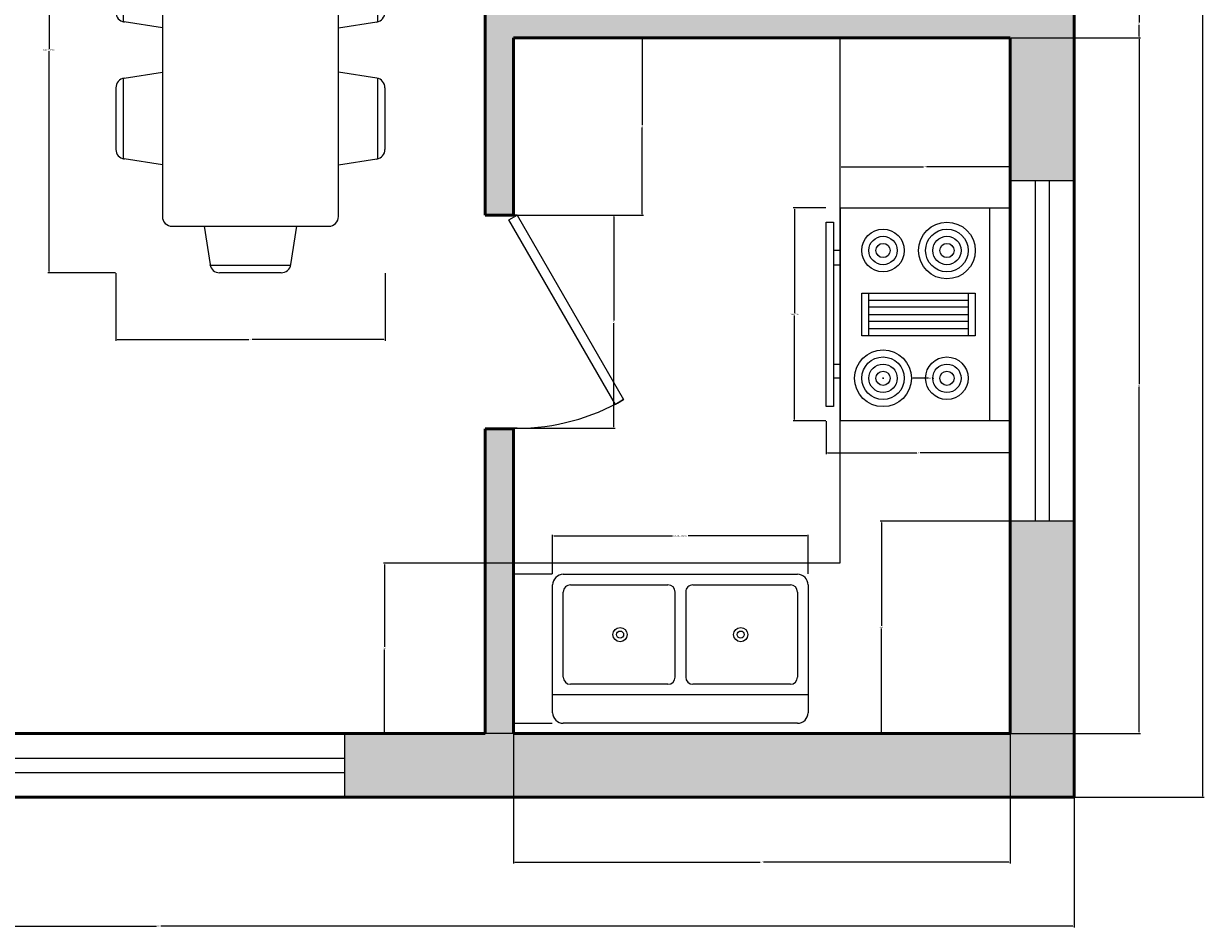
# Model space of a CAD drawing. Units: inches. Extents: x 2130 to 2425, y 2862 to 3216.
# Tile 2 of 4: x 2259 to 2425, y 2862 to 2989. Entities that reach past the tile are written whole.
import ezdxf

# ---------------------------------------------------------------- set-up
doc = ezdxf.new("R2010")
doc.units = ezdxf.units.IN
for name, color, linetype, lineweight in [('A-ANNO-DIMS', 2, 'Continuous', 18), ('A-DOOR', 3, 'Continuous', 25), ('A-EQPM', 8, 'Continuous', 25), ('A-FLOR-CASE', 9, 'Continuous', 25), ('A-FLOR-FIXT', 9, 'Continuous', 18), ('A-FURN', 8, 'Continuous', 18), ('A-GLAZ', 4, 'Continuous', 18), ('A-WALL', 7, 'Continuous', 50), ('A-WALL-PATT', 18, 'Continuous', 13)]:
    doc.layers.add(name, color=color, linetype=linetype, lineweight=lineweight)
doc.styles.get("Standard").update_dxf_attribs({"font": 'arial.ttf'})
doc.dimstyles.get("Standard").update_dxf_attribs({"dimtxt": 0.18, "dimasz": 0.18, "dimexe": 0.18, "dimexo": 0.0625, "dimgap": 0.09, "dimtad": 0, "dimtih": 1, "dimtoh": 1, "dimdec": 4, "dimzin": 0, "dimdsep": 46, "dimtxsty": 'Standard', "dimcen": 0.09, "dimadec": 0, "dimazin": 0, "dimtfac": 1, "dimtdec": 4, "dimtofl": 0, "dimtmove": 0, "dimatfit": 3, "dimfxl": 1, "dimtolj": 1, "dimtzin": 0, "dimarcsym": 0})

# ---------------------------------------------------------------- blocks, each defined once
blk = doc.blocks.new('Dining Set - 36 x 72 in.')
for p, q in [((-20.29, 27.5), (-7.71, 27.5)), ((7.71, 27.5), (20.29, 27.5)), ((-22.26, 25.81), (-23.48, 18)), ((-22.23, 26), (-5.76, 26)), ((-4.52, 18), (-5.74, 25.81)), ((5.74, 25.81), (4.52, 18)), ((5.77, 26), (22.24, 26)), ((23.48, 18), (22.26, 25.81)), ((34, 18), (-34, 18)), ((-36, 16), (-36, -16)), ((36, -16), (36, 16)), ((-44, 8.23), (-44, -8.24)), ((-43.81, 8.26), (-36, 9.48)), ((43.81, 8.26), (36, 9.48)), ((44, 8.23), (44, -8.24)), ((-45.5, 6.29), (-45.5, -6.29)), ((45.5, 6.29), (45.5, -6.29)), ((-36, -9.48), (-43.81, -8.26)), ((36, -9.48), (43.81, -8.26)), ((-34, -18), (34, -18)), ((-22.26, -25.81), (-23.48, -18)), ((-4.52, -18), (-5.74, -25.81)), ((5.74, -25.81), (4.52, -18)), ((23.48, -18), (22.26, -25.81)), ((-22.23, -26), (-5.76, -26)), ((5.77, -26), (22.24, -26)), ((-20.29, -27.5), (-7.71, -27.5)), ((7.71, -27.5), (20.29, -27.5))]:
    blk.add_line(p, q)
for centre, start, end in [((-20.29, 25.5), 90, 171.1198), ((-7.71, 25.5), 8.881, 90), ((7.71, 25.5), 90, 171.1198), ((20.29, 25.5), 8.881, 90), ((-34, 16), 90, 180), ((34, 16), 0, 90), ((-43.5, 6.29), 98.8806, 180), ((43.5, 6.29), 0, 81.1194), ((-43.5, -6.29), 180, 261.1194), ((43.5, -6.29), 278.8806, 0), ((-34, -16), 180, 270), ((34, -16), 270, 0), ((-20.29, -25.5), 188.8802, 270), ((-7.71, -25.5), 270, 351.1191), ((7.71, -25.5), 188.8802, 270), ((20.29, -25.5), 270, 351.1191)]:
    blk.add_arc(centre, 2, start, end)
blk = doc.blocks.new('Range-Oven - 30 in top')
for p, q in [((0, -3), (30, -3)), ((12, -6), (18, -6)), ((13, -20), (13, -6)), ((14, -6), (14, -20)), ((15, -20), (15, -6)), ((16, -6), (16, -20)), ((17, -20), (17, -6)), ((18, -20), (12, -20)), ((6, -24), (6, -25)), ((8, -25), (8, -24)), ((22, -25), (22, -24)), ((24, -24), (24, -25))]:
    blk.add_line(p, q)
for points in [[(0, -24), (0, 0), (30, 0), (30, -24)], [(12, -21), (12, -5), (18, -5), (18, -21)], [(2, -26), (2, -25), (28, -25), (28, -26)]]:
    blk.add_lwpolyline(points, close=True)
for centre, radius in [((6, -9), 4), ((6, -9), 3), ((24, -9), 3), ((6, -9), 2), ((6, -9), 1), ((24, -9), 2), ((24, -9), 1), ((24, -18), 4), ((6, -18), 3), ((6, -18), 2), ((24, -18), 3), ((24, -18), 2), ((6, -18), 1), ((24, -18), 1)]:
    blk.add_circle(centre, radius)
blk = doc.blocks.new('Sink-double - 36 in top')
for p, q in [((-18, -4), (18, -4)), ((-0.75, -18.5), (-0.75, -6.5)), ((0.75, -6.5), (0.75, -18.5))]:
    blk.add_line(p, q)
for points in [[(-16.5, 0), (16.5, 0)], [(-18, -19.5), (-18, -1.5)], [(18, -1.5), (18, -19.5)], [(-16.5, -18.5), (-16.5, -6.5)], [(-15.5, -5.5), (-1.75, -5.5)], [(1.75, -5.5), (15.5, -5.5)], [(16.5, -6.5), (16.5, -18.5)], [(-1.75, -19.5), (-15.5, -19.5)], [(15.5, -19.5), (1.75, -19.5)], [(16.5, -21), (-16.5, -21)]]:
    blk.add_lwpolyline(points)
for centre, radius in [((-8.5, -12.5), 1), ((8.5, -12.5), 1), ((-8.5, -12.5), 0.5), ((8.5, -12.5), 0.5)]:
    blk.add_circle(centre, radius)
for centre, radius, start, end in [((-16.5, -1.5), 1.5, 90, 180), ((16.5, -1.5), 1.5, 0, 90), ((-15.5, -6.5), 1, 90, 180), ((-1.75, -6.5), 1, 0, 90), ((1.75, -6.5), 1, 90, 180), ((15.5, -6.5), 1, 0, 90), ((-16.5, -19.5), 1.5, 180, 270), ((-15.5, -18.5), 1, 180, 270), ((-1.75, -18.5), 1, 270, 0), ((1.75, -18.5), 1, 180, 270), ((15.5, -18.5), 1, 270, 0), ((16.5, -19.5), 1.5, 270, 0)]:
    blk.add_arc(centre, radius, start, end)
blk = doc.blocks.new('*U10')
for p, q in [((0, 0), (0, -6)), ((40, 0), (40, -6))]:
    blk.add_line(p, q)
blk.add_lwpolyline([(0, 0), (34.64, 20), (35.52, 18.48), (0.87, -1.52)], close=True)
blk.add_arc((0, 0), 40, 0, 30)
blk = doc.blocks.new('WIN-48IN')
for p, q in [((0, 0), (0, 9)), ((48, 9), (48, 0)), ((0, 5.5), (48, 5.5)), ((0, 3.5), (48, 3.5))]:
    blk.add_line(p, q)
blk = doc.blocks.new('*D29')
at = {"layer": 'A-ANNO-DIMS', "color": 0, "lineweight": -2, "transparency": 16777216}
for p, q in [((2271.46, 3016.6), (2261.94, 3016.6)), ((2262.12, 3016.42), (2262.12, 2985.41)), ((2262.12, 2954.04), (2262.12, 2985.05)), ((2271.46, 2953.86), (2261.94, 2953.86))]:
    blk.add_line(p, q, dxfattribs=at)
at = {"layer": 'A-ANNO-DIMS', "color": 0, "transparency": 16777216}
for points in [[(2262.09, 3016.42), (2262.15, 3016.42), (2262.12, 3016.6)], [(2262.09, 2954.04), (2262.15, 2954.04), (2262.12, 2953.86)]]:
    blk.add_solid(points, dxfattribs=at)
at = {"layer": 'Defpoints', "color": 0, "transparency": 16777216}
for p in [(2271.53, 3016.6), (2262.12, 2953.86), (2271.53, 2953.86)]:
    blk.add_point(p, dxfattribs=at)
at = {"layer": 'A-ANNO-DIMS', "color": 0, "transparency": 16777216, "insert": (2262.12, 2985.23), "char_height": 0.18, "attachment_point": 5}
blk.add_mtext('\\A1;DINING SET 63', dxfattribs=at)
blk = doc.blocks.new('*D30')
at = {"layer": 'A-ANNO-DIMS', "color": 0, "lineweight": -2, "transparency": 16777216}
for p, q in [((2271.53, 2953.8), (2271.53, 2944.27)), ((2309.45, 2953.8), (2309.45, 2944.27)), ((2271.71, 2944.45), (2290.27, 2944.45)), ((2309.27, 2944.45), (2290.71, 2944.45))]:
    blk.add_line(p, q, dxfattribs=at)
at = {"layer": 'A-ANNO-DIMS', "color": 0, "transparency": 16777216}
for points in [[(2271.71, 2944.48), (2271.71, 2944.42), (2271.53, 2944.45)], [(2309.27, 2944.48), (2309.27, 2944.42), (2309.45, 2944.45)]]:
    blk.add_solid(points, dxfattribs=at)
at = {"layer": 'Defpoints', "color": 0, "transparency": 16777216}
for p in [(2271.53, 2953.86), (2309.45, 2953.86), (2309.45, 2944.45)]:
    blk.add_point(p, dxfattribs=at)
at = {"layer": 'A-ANNO-DIMS', "color": 0, "transparency": 16777216, "insert": (2290.49, 2944.45), "char_height": 0.18, "attachment_point": 5}
blk.add_mtext('\\A1;38', dxfattribs=at)
blk = doc.blocks.new('*D31')
at = {"layer": 'A-ANNO-DIMS', "color": 0, "lineweight": -2, "transparency": 16777216}
for p, q in [((2371.56, 2962.99), (2366.95, 2962.99)), ((2367.13, 2962.81), (2367.13, 2948.17)), ((2367.13, 2933.17), (2367.13, 2947.81)), ((2371.56, 2932.99), (2366.95, 2932.99))]:
    blk.add_line(p, q, dxfattribs=at)
at = {"layer": 'A-ANNO-DIMS', "color": 0, "transparency": 16777216}
for points in [[(2367.1, 2962.81), (2367.16, 2962.81), (2367.13, 2962.99)], [(2367.1, 2933.17), (2367.16, 2933.17), (2367.13, 2932.99)]]:
    blk.add_solid(points, dxfattribs=at)
at = {"layer": 'Defpoints', "color": 0, "transparency": 16777216}
for p in [(2371.63, 2962.99), (2367.13, 2932.99), (2371.63, 2932.99)]:
    blk.add_point(p, dxfattribs=at)
at = {"layer": 'A-ANNO-DIMS', "color": 0, "transparency": 16777216, "insert": (2367.13, 2947.99), "char_height": 0.18, "attachment_point": 5}
blk.add_mtext('\\A1;RANGE 30', dxfattribs=at)
blk = doc.blocks.new('*D32')
at = {"layer": 'A-ANNO-DIMS', "color": 0, "lineweight": -2, "transparency": 16777216}
for p, q in [((2371.63, 2932.93), (2371.63, 2928.31)), ((2397.63, 2932.93), (2397.63, 2928.31)), ((2371.81, 2928.49), (2384.4, 2928.49)), ((2397.45, 2928.49), (2384.85, 2928.49))]:
    blk.add_line(p, q, dxfattribs=at)
at = {"layer": 'A-ANNO-DIMS', "color": 0, "transparency": 16777216}
for points in [[(2371.81, 2928.52), (2371.81, 2928.46), (2371.63, 2928.49)], [(2397.45, 2928.52), (2397.45, 2928.46), (2397.63, 2928.49)]]:
    blk.add_solid(points, dxfattribs=at)
at = {"layer": 'Defpoints', "color": 0, "transparency": 16777216}
for p in [(2371.63, 2932.99), (2397.63, 2932.99), (2397.63, 2928.49)]:
    blk.add_point(p, dxfattribs=at)
at = {"layer": 'A-ANNO-DIMS', "color": 0, "transparency": 16777216, "insert": (2384.63, 2928.49), "char_height": 0.18, "attachment_point": 5}
blk.add_mtext('\\A1;26', dxfattribs=at)
blk = doc.blocks.new('*D33')
at = {"layer": 'A-ANNO-DIMS', "color": 0, "lineweight": -2, "transparency": 16777216}
for p, q in [((2333.07, 2911.44), (2333.07, 2916.95)), ((2333.25, 2916.77), (2349.98, 2916.77)), ((2368.89, 2916.77), (2352.17, 2916.77)), ((2369.07, 2911.44), (2369.07, 2916.95))]:
    blk.add_line(p, q, dxfattribs=at)
at = {"layer": 'A-ANNO-DIMS', "color": 0, "transparency": 16777216}
for points in [[(2333.25, 2916.8), (2333.25, 2916.74), (2333.07, 2916.77)], [(2368.89, 2916.8), (2368.89, 2916.74), (2369.07, 2916.77)]]:
    blk.add_solid(points, dxfattribs=at)
at = {"layer": 'Defpoints', "color": 0, "transparency": 16777216}
for p in [(2333.07, 2916.77), (2333.07, 2911.37), (2369.07, 2911.37)]:
    blk.add_point(p, dxfattribs=at)
at = {"layer": 'A-ANNO-DIMS', "color": 0, "transparency": 16777216, "insert": (2351.07, 2916.77), "char_height": 0.18, "attachment_point": 5}
blk.add_mtext('\\A1;DOUBLE SINK 36', dxfattribs=at)
blk = doc.blocks.new('*D34')
at = {"layer": 'A-ANNO-DIMS', "color": 0, "lineweight": -2, "transparency": 16777216}
for p, q in [((2333.01, 2911.37), (2327.49, 2911.37)), ((2327.67, 2911.19), (2327.67, 2901.06)), ((2327.67, 2890.55), (2327.67, 2900.69)), ((2333.01, 2890.37), (2327.49, 2890.37))]:
    blk.add_line(p, q, dxfattribs=at)
at = {"layer": 'A-ANNO-DIMS', "color": 0, "transparency": 16777216}
for points in [[(2327.64, 2911.19), (2327.7, 2911.19), (2327.67, 2911.37)], [(2327.64, 2890.55), (2327.7, 2890.55), (2327.67, 2890.37)]]:
    blk.add_solid(points, dxfattribs=at)
at = {"layer": 'Defpoints', "color": 0, "transparency": 16777216}
for p in [(2333.07, 2911.37), (2327.67, 2890.37), (2333.07, 2890.37)]:
    blk.add_point(p, dxfattribs=at)
at = {"layer": 'A-ANNO-DIMS', "color": 0, "transparency": 16777216, "insert": (2327.67, 2900.87), "char_height": 0.18, "attachment_point": 5}
blk.add_mtext('\\A1;21', dxfattribs=at)
blk = doc.blocks.new('*D35')
at = {"layer": 'A-ANNO-DIMS', "color": 0, "lineweight": -2, "transparency": 16777216}
for p, q in [((2148.55, 2879.89), (2148.55, 2861.62)), ((2406.55, 2879.89), (2406.55, 2861.62)), ((2148.73, 2861.8), (2277.26, 2861.8)), ((2406.37, 2861.8), (2277.84, 2861.8))]:
    blk.add_line(p, q, dxfattribs=at)
at = {"layer": 'A-ANNO-DIMS', "color": 0, "transparency": 16777216}
for points in [[(2148.73, 2861.83), (2148.73, 2861.77), (2148.55, 2861.8)], [(2406.37, 2861.83), (2406.37, 2861.77), (2406.55, 2861.8)]]:
    blk.add_solid(points, dxfattribs=at)
at = {"layer": 'Defpoints', "color": 0, "transparency": 16777216}
for p in [(2148.55, 2879.95), (2406.55, 2879.95), (2406.55, 2861.8)]:
    blk.add_point(p, dxfattribs=at)
at = {"layer": 'A-ANNO-DIMS', "color": 0, "transparency": 16777216, "insert": (2277.55, 2861.8), "char_height": 0.18, "attachment_point": 5}
blk.add_mtext('\\A1;258', dxfattribs=at)
blk = doc.blocks.new('*D36')
at = {"layer": 'A-ANNO-DIMS', "color": 0, "lineweight": -2, "transparency": 16777216}
for p, q in [((2406.61, 3197.95), (2424.88, 3197.95)), ((2424.7, 3197.77), (2424.7, 3039.14)), ((2424.7, 2880.13), (2424.7, 3038.77)), ((2406.61, 2879.95), (2424.88, 2879.95))]:
    blk.add_line(p, q, dxfattribs=at)
at = {"layer": 'A-ANNO-DIMS', "color": 0, "transparency": 16777216}
for points in [[(2424.67, 3197.77), (2424.73, 3197.77), (2424.7, 3197.95)], [(2424.67, 2880.13), (2424.73, 2880.13), (2424.7, 2879.95)]]:
    blk.add_solid(points, dxfattribs=at)
at = {"layer": 'Defpoints', "color": 0, "transparency": 16777216}
for p in [(2406.55, 3197.95), (2424.7, 3197.95), (2406.55, 2879.95)]:
    blk.add_point(p, dxfattribs=at)
at = {"layer": 'A-ANNO-DIMS', "color": 0, "transparency": 16777216, "insert": (2424.7, 3038.95), "char_height": 0.18, "attachment_point": 5}
blk.add_mtext('\\A1;318', dxfattribs=at)
blk = doc.blocks.new('*D42')
at = {"layer": 'A-ANNO-DIMS', "color": 0, "lineweight": -2, "transparency": 16777216}
for p, q in [((2397.49, 2918.86), (2379.22, 2918.86)), ((2379.4, 2918.68), (2379.4, 2904.09)), ((2379.4, 2889.13), (2379.4, 2903.72)), ((2397.49, 2888.95), (2379.22, 2888.95))]:
    blk.add_line(p, q, dxfattribs=at)
at = {"layer": 'A-ANNO-DIMS', "color": 0, "transparency": 16777216}
for points in [[(2379.37, 2918.68), (2379.43, 2918.68), (2379.4, 2918.86)], [(2379.37, 2889.13), (2379.43, 2889.13), (2379.4, 2888.95)]]:
    blk.add_solid(points, dxfattribs=at)
at = {"layer": 'Defpoints', "color": 0, "transparency": 16777216}
for p in [(2379.4, 2918.86), (2397.55, 2918.86), (2397.55, 2888.95)]:
    blk.add_point(p, dxfattribs=at)
at = {"layer": 'A-ANNO-DIMS', "color": 0, "transparency": 16777216, "insert": (2379.4, 2903.91), "char_height": 0.18, "attachment_point": 5}
blk.add_mtext('\\A1;29.9', dxfattribs=at)
blk = doc.blocks.new('*D53')
at = {"layer": 'A-ANNO-DIMS', "color": 0, "lineweight": -2, "transparency": 16777216}
for p, q in [((2327.55, 2888.89), (2327.55, 2870.62)), ((2397.55, 2888.89), (2397.55, 2870.62)), ((2327.73, 2870.8), (2362.33, 2870.8)), ((2397.37, 2870.8), (2362.77, 2870.8))]:
    blk.add_line(p, q, dxfattribs=at)
at = {"layer": 'A-ANNO-DIMS', "color": 0, "transparency": 16777216}
for points in [[(2327.73, 2870.83), (2327.73, 2870.77), (2327.55, 2870.8)], [(2397.37, 2870.83), (2397.37, 2870.77), (2397.55, 2870.8)]]:
    blk.add_solid(points, dxfattribs=at)
at = {"layer": 'Defpoints', "color": 0, "transparency": 16777216}
for p in [(2327.55, 2888.95), (2397.55, 2888.95), (2327.55, 2870.8)]:
    blk.add_point(p, dxfattribs=at)
at = {"layer": 'A-ANNO-DIMS', "color": 0, "transparency": 16777216, "insert": (2362.55, 2870.8), "char_height": 0.18, "attachment_point": 5}
blk.add_mtext('\\A1;70', dxfattribs=at)
blk = doc.blocks.new('*D55')
at = {"layer": 'A-ANNO-DIMS', "color": 0, "lineweight": -2, "transparency": 16777216}
for p, q in [((2397.612727, 2990.954394), (2415.880227, 2990.954394)), ((2415.700227, 2990.774394), (2415.700227, 2989.134394)), ((2415.700227, 2987.134394), (2415.700227, 2988.774394)), ((2397.612727, 2986.954394), (2415.880227, 2986.954394))]:
    blk.add_line(p, q, dxfattribs=at)
at = {"layer": 'A-ANNO-DIMS', "color": 0, "transparency": 16777216}
for points in [[(2415.670227, 2990.774394), (2415.730227, 2990.774394), (2415.700227, 2990.954394)], [(2415.670227, 2987.134394), (2415.730227, 2987.134394), (2415.700227, 2986.954394)]]:
    blk.add_solid(points, dxfattribs=at)
at = {"layer": 'Defpoints', "color": 0, "transparency": 16777216}
for p in [(2397.550227, 2990.954394), (2397.550227, 2986.954394), (2415.700227, 2986.954394)]:
    blk.add_point(p, dxfattribs=at)
at = {"layer": 'A-ANNO-DIMS', "color": 0, "transparency": 16777216, "insert": (2415.700227, 2988.954394), "char_height": 0.18, "attachment_point": 5}
blk.add_mtext('\\A1;4', dxfattribs=at)
blk = doc.blocks.new('*D56')
at = {"layer": 'A-ANNO-DIMS', "color": 0, "lineweight": -2, "transparency": 16777216}
for p, q in [((2397.61, 2986.95), (2415.88, 2986.95)), ((2415.7, 2986.77), (2415.7, 2938.14)), ((2415.7, 2889.13), (2415.7, 2937.77)), ((2397.61, 2888.95), (2415.88, 2888.95))]:
    blk.add_line(p, q, dxfattribs=at)
at = {"layer": 'A-ANNO-DIMS', "color": 0, "transparency": 16777216}
for points in [[(2415.67, 2986.77), (2415.73, 2986.77), (2415.7, 2986.95)], [(2415.67, 2889.13), (2415.73, 2889.13), (2415.7, 2888.95)]]:
    blk.add_solid(points, dxfattribs=at)
at = {"layer": 'Defpoints', "color": 0, "transparency": 16777216}
for p in [(2397.55, 2986.95), (2397.55, 2888.95), (2415.7, 2888.95)]:
    blk.add_point(p, dxfattribs=at)
at = {"layer": 'A-ANNO-DIMS', "color": 0, "transparency": 16777216, "insert": (2415.7, 2937.95), "char_height": 0.18, "attachment_point": 5}
blk.add_mtext('\\A1;98', dxfattribs=at)
blk = doc.blocks.new('*D65')
at = {"layer": 'A-ANNO-DIMS', "color": 0, "lineweight": -2, "transparency": 16777216}
for p, q in [((2323.61, 2961.95), (2341.88, 2961.95)), ((2341.7, 2961.77), (2341.7, 2947.14)), ((2341.7, 2932.13), (2341.7, 2946.77)), ((2323.61, 2931.95), (2341.88, 2931.95))]:
    blk.add_line(p, q, dxfattribs=at)
at = {"layer": 'A-ANNO-DIMS', "color": 0, "transparency": 16777216}
for points in [[(2341.67, 2961.77), (2341.73, 2961.77), (2341.7, 2961.95)], [(2341.67, 2932.13), (2341.73, 2932.13), (2341.7, 2931.95)]]:
    blk.add_solid(points, dxfattribs=at)
at = {"layer": 'Defpoints', "color": 0, "transparency": 16777216}
for p in [(2323.55, 2961.95), (2323.55, 2931.95), (2341.7, 2931.95)]:
    blk.add_point(p, dxfattribs=at)
at = {"layer": 'A-ANNO-DIMS', "color": 0, "transparency": 16777216, "insert": (2341.7, 2946.95), "char_height": 0.18, "attachment_point": 5}
blk.add_mtext('\\A1;30', dxfattribs=at)
blk = doc.blocks.new('*D66')
at = {"layer": 'A-ANNO-DIMS', "color": 0, "lineweight": -2, "transparency": 16777216}
for p, q in [((2327.61, 2986.95), (2345.88, 2986.95)), ((2345.7, 2986.77), (2345.7, 2974.64)), ((2345.7, 2962.13), (2345.7, 2974.27)), ((2327.61, 2961.95), (2345.88, 2961.95))]:
    blk.add_line(p, q, dxfattribs=at)
at = {"layer": 'A-ANNO-DIMS', "color": 0, "transparency": 16777216}
for points in [[(2345.67, 2986.77), (2345.73, 2986.77), (2345.7, 2986.95)], [(2345.67, 2962.13), (2345.73, 2962.13), (2345.7, 2961.95)]]:
    blk.add_solid(points, dxfattribs=at)
at = {"layer": 'Defpoints', "color": 0, "transparency": 16777216}
for p in [(2327.55, 2986.95), (2327.55, 2961.95), (2345.7, 2961.95)]:
    blk.add_point(p, dxfattribs=at)
at = {"layer": 'A-ANNO-DIMS', "color": 0, "transparency": 16777216, "insert": (2345.7, 2974.45), "char_height": 0.18, "attachment_point": 5}
blk.add_mtext('\\A1;25', dxfattribs=at)
blk = doc.blocks.new('*D71')
at = {"layer": 'A-ANNO-DIMS', "color": 0, "lineweight": -2, "transparency": 16777216}
for p, q in [((2373.55, 2986.89), (2373.55, 2968.62)), ((2397.55, 2986.89), (2397.55, 2968.62)), ((2373.73, 2968.8), (2385.33, 2968.8)), ((2397.37, 2968.8), (2385.77, 2968.8))]:
    blk.add_line(p, q, dxfattribs=at)
at = {"layer": 'A-ANNO-DIMS', "color": 0, "transparency": 16777216}
for points in [[(2373.73, 2968.83), (2373.73, 2968.77), (2373.55, 2968.8)], [(2397.37, 2968.83), (2397.37, 2968.77), (2397.55, 2968.8)]]:
    blk.add_solid(points, dxfattribs=at)
at = {"layer": 'Defpoints', "color": 0, "transparency": 16777216}
for p in [(2373.55, 2986.95), (2397.55, 2986.95), (2373.55, 2968.8)]:
    blk.add_point(p, dxfattribs=at)
at = {"layer": 'A-ANNO-DIMS', "color": 0, "transparency": 16777216, "insert": (2385.55, 2968.8), "char_height": 0.18, "attachment_point": 5}
blk.add_mtext('\\A1;24', dxfattribs=at)
blk = doc.blocks.new('*D72')
at = {"layer": 'A-ANNO-DIMS', "color": 0, "lineweight": -2, "transparency": 16777216}
for p, q in [((2327.49, 2912.95), (2309.22, 2912.95)), ((2309.4, 2912.77), (2309.4, 2901.13)), ((2309.4, 2889.13), (2309.4, 2900.77)), ((2327.49, 2888.95), (2309.22, 2888.95))]:
    blk.add_line(p, q, dxfattribs=at)
at = {"layer": 'A-ANNO-DIMS', "color": 0, "transparency": 16777216}
for points in [[(2309.37, 2912.77), (2309.43, 2912.77), (2309.4, 2912.95)], [(2309.37, 2889.13), (2309.43, 2889.13), (2309.4, 2888.95)]]:
    blk.add_solid(points, dxfattribs=at)
at = {"layer": 'Defpoints', "color": 0, "transparency": 16777216}
for p in [(2309.4, 2912.95), (2327.55, 2912.95), (2327.55, 2888.95)]:
    blk.add_point(p, dxfattribs=at)
at = {"layer": 'A-ANNO-DIMS', "color": 0, "transparency": 16777216, "insert": (2309.4, 2900.95), "char_height": 0.18, "attachment_point": 5}
blk.add_mtext('\\A1;24', dxfattribs=at)
blk = doc.blocks.new('*D73')
at = {"layer": 'A-ANNO-DIMS', "color": 0, "lineweight": -2, "transparency": 16777216}
for p, q in [((2379.54, 2938.99), (2379.72, 2938.99)), ((2379.63, 2938.9), (2379.63, 2939.08)), ((2386.03, 2938.99), (2383.81, 2938.99))]:
    blk.add_line(p, q, dxfattribs=at)
at = {"layer": 'A-ANNO-DIMS', "color": 0, "transparency": 16777216}
blk.add_solid([(2383.81, 2939.02), (2383.81, 2938.96), (2383.63, 2938.99)], dxfattribs=at)
at = {"layer": 'Defpoints', "color": 0, "transparency": 16777216}
for p in [(2375.63, 2938.99), (2383.63, 2938.99)]:
    blk.add_point(p, dxfattribs=at)
at = {"layer": 'A-ANNO-DIMS', "color": 0, "transparency": 16777216, "insert": (2386.46, 2938.99), "char_height": 0.18, "attachment_point": 5}
blk.add_mtext('\\A1;2X ∅8', dxfattribs=at)

msp = doc.modelspace()

# ---------------------------------------------------------------- hatches: boundary and pattern name
at = {"layer": 'A-WALL-PATT'}
h = msp.add_hatch(color=256, dxfattribs=at)
h.dxf.hatch_style = 1
h.paths.add_polyline_path([(2406.5502, 3197.9544), (2367.6433, 3197.9544), (2367.6433, 3188.9544), (2397.5502, 3188.9544), (2397.5502, 3068.9544), (2325.5502, 3068.9544), (2317.5502, 3068.9544), (2317.5502, 3064.9544), (2323.5502, 3064.9544), (2323.5502, 3056.9544), (2327.5502, 3056.9544), (2327.5502, 3064.9544), (2397.5502, 3064.9544), (2397.5502, 2990.9544), (2327.5502, 2990.9544), (2327.5502, 3032.9544), (2323.5502, 3032.9544), (2323.5502, 2986.9544), (2323.5502, 2961.9544), (2327.5502, 2961.9544), (2327.5502, 2986.9544), (2397.5502, 2986.9544), (2397.5502, 2966.8556), (2406.5502, 2966.8556)])
h = msp.add_hatch(color=256, dxfattribs=at)
h.dxf.hatch_style = 1
h.paths.add_polyline_path([(2406.5502, 2918.8556), (2397.5502, 2918.8556), (2397.5502, 2888.9544), (2327.5502, 2888.9544), (2327.5502, 2913.9544), (2327.5502, 2931.8784), (2323.5502, 2931.8784), (2323.5502, 2913.9544), (2323.5502, 2888.9544), (2303.7452, 2888.9544), (2303.7452, 2879.9544), (2406.5502, 2879.9544)])

# ---------------------------------------------------------------- linework, layer by layer
at = {"layer": 'A-FLOR-CASE'}
for p, q in [((2373.5502, 2986.9544), (2373.5502, 2912.9544)), ((2373.5502, 2912.9544), (2327.5502, 2912.9544))]:
    msp.add_line(p, q, dxfattribs=at)
at = {"layer": 'A-WALL'}
for p, q in [((2323.5502, 3032.9544), (2323.5502, 2986.9544)), ((2323.5502, 2986.9544), (2323.5502, 2961.9544)), ((2327.5502, 2986.9544), (2397.5502, 2986.9544)), ((2327.5502, 2986.9544), (2327.5502, 2961.9544)), ((2397.5502, 2986.9544), (2397.5502, 2888.9544)), ((2327.5502, 2961.9544), (2323.5502, 2961.9544)), ((2327.5502, 2931.8784), (2323.5502, 2931.8784)), ((2323.5502, 2931.8784), (2323.5502, 2913.9544)), ((2327.5502, 2913.9544), (2327.5502, 2931.8784)), ((2323.5502, 2913.9544), (2323.5502, 2888.9544)), ((2327.5502, 2913.9544), (2327.5502, 2888.9544)), ((2323.5502, 2888.9544), (2211.5502, 2888.9544)), ((2397.5502, 2888.9544), (2327.5502, 2888.9544))]:
    msp.add_line(p, q, dxfattribs=at)
msp.add_lwpolyline([(2163.5502, 2879.9544), (2148.5502, 2879.9544), (2148.5502, 3197.9544), (2406.5502, 3197.9544), (2406.5502, 2879.9544), (2211.5502, 2879.9544)], dxfattribs=at)

# ---------------------------------------------------------------- block references
at = {"layer": 'A-DOOR', "xscale": 0.75, "yscale": 0.75, "zscale": 0.75, "rotation": 270}
msp.add_blockref('*U10', (2328.0502, 2961.9544), dxfattribs=at)
at = {"layer": 'A-EQPM', "rotation": 270}
msp.add_blockref('Range-Oven - 30 in top', (2397.6253, 2962.9882), dxfattribs=at)
at = {"layer": 'A-FLOR-FIXT', "rotation": 180}
msp.add_blockref('Sink-double - 36 in top', (2351.073, 2890.3749), dxfattribs=at)
at = {"layer": 'A-FURN', "xscale": 0.6894662824826121, "yscale": 0.6894662824826121, "zscale": 0.6894662824826121, "rotation": 270}
msp.add_blockref('Dining Set - 36 x 72 in.', (2290.487, 2985.2285), dxfattribs=at)
at = {"layer": 'A-GLAZ', "rotation": 269.9999999999989}
msp.add_blockref('WIN-48IN', (2397.5498, 2966.8554), dxfattribs=at)
at = {"layer": 'A-GLAZ'}
msp.add_blockref('WIN-48IN', (2255.7454, 2879.954), dxfattribs=at)

# ---------------------------------------------------------------- dimensions: what is measured, and where the dimension line sits
at = {"layer": 'A-ANNO-DIMS'}
for base, p1, p2, angle, override, picture, middle in [((2424.7002, 3197.9544), (2406.5502, 2879.9544), (2406.5502, 3197.9544), 90, {"dimdec": 0, "dimlfac": 1, "dimrnd": 0, "dimzin": 0, "dimdsep": 46, "dimlunit": 2}, '*D36', (2424.7002, 3038.9544)), ((2415.7002, 2986.9544), (2397.5502, 2990.9544), (2397.5502, 2986.9544), 270, {"dimdec": 0, "dimlfac": 1, "dimrnd": 0, "dimzin": 0, "dimdsep": 46, "dimlunit": 2}, '*D55', (2415.7002, 2988.9544)), ((2345.7002, 2961.9544), (2327.5502, 2986.9544), (2327.5502, 2961.9544), 270, {"dimdec": 0, "dimlfac": 1, "dimrnd": 0, "dimzin": 0, "dimdsep": 46, "dimlunit": 2}, '*D66', (2345.7002, 2974.4544)), ((2373.5502, 2968.8044), (2397.5502, 2986.9544), (2373.5502, 2986.9544), 180, {"dimdec": 0, "dimlfac": 1, "dimrnd": 0, "dimzin": 0, "dimdsep": 46, "dimlunit": 2}, '*D71', (2385.5502, 2968.8044)), ((2415.7002, 2888.9544), (2397.5502, 2986.9544), (2397.5502, 2888.9544), 270, {"dimdec": 0, "dimlfac": 1, "dimrnd": 0, "dimzin": 0, "dimdsep": 46, "dimlunit": 2}, '*D56', (2415.7002, 2937.9544)), ((2341.7002, 2931.9544), (2323.5502, 2961.9544), (2323.5502, 2931.9544), 270, {"dimdec": 0, "dimlfac": 1, "dimrnd": 0, "dimzin": 0, "dimdsep": 46, "dimlunit": 2}, '*D65', (2341.7002, 2946.9544)), ((2379.4002, 2918.8556), (2397.5502, 2888.9544), (2397.5502, 2918.8556), 90, {"dimdec": 1, "dimlfac": 1, "dimrnd": 0, "dimzin": 0, "dimdsep": 46, "dimlunit": 2}, '*D42', (2379.4002, 2903.905)), ((2309.4002, 2912.9544), (2327.5502, 2888.9544), (2327.5502, 2912.9544), 90, {"dimdec": 0, "dimlfac": 1, "dimrnd": 0, "dimzin": 0, "dimdsep": 46, "dimlunit": 2}, '*D72', (2309.4002, 2900.9544)), ((2327.673, 2890.3749), (2333.073, 2911.3749), (2333.073, 2890.3749), 270, {"dimdec": 0, "dimlfac": 1, "dimrnd": 0, "dimzin": 0, "dimdsep": 46, "dimlunit": 2}, '*D34', (2327.673, 2900.8749)), ((2327.5502, 2870.8044), (2397.5502, 2888.9544), (2327.5502, 2888.9544), 180, {"dimdec": 0, "dimlfac": 1, "dimrnd": 0, "dimzin": 0, "dimdsep": 46, "dimlunit": 2}, '*D53', (2362.5502, 2870.8044))]:
    dim = msp.add_linear_dim(base=base, p1=p1, p2=p2, angle=angle, dimstyle='Standard', override=override, dxfattribs=at)
    dim.commit()
    dim.dimension.update_dxf_attribs({"geometry": picture, "text_midpoint": middle})
for base, p1, p2, angle, text, picture, middle in [((2262.1154, 2953.8578), (2271.5266, 3016.5993), (2271.5266, 2953.8578), 270, 'DINING SET <>', '*D29', (2262.1154, 2985.2285)), ((2367.1253, 2932.9882), (2371.6253, 2962.9882), (2371.6253, 2932.9882), 270, 'RANGE <>', '*D31', (2367.1253, 2947.9882)), ((2333.073, 2916.7749), (2369.073, 2911.3749), (2333.073, 2911.3749), 180, 'DOUBLE SINK <>', '*D33', (2351.073, 2916.7749))]:
    dim = msp.add_linear_dim(base=base, p1=p1, p2=p2, angle=angle, text=text, dimstyle='Standard', override={"dimdec": 0, "dimlfac": 1, "dimrnd": 0, "dimzin": 0, "dimdsep": 46, "dimlunit": 2}, dxfattribs=at)
    dim.commit()
    dim.dimension.update_dxf_attribs({"geometry": picture, "text_midpoint": middle})
for base, p1, p2, picture, middle in [((2309.4473, 2944.4466), (2271.5266, 2953.8578), (2309.4473, 2953.8578), '*D30', (2290.487, 2944.4466)), ((2397.6253, 2928.4882), (2371.6253, 2932.9882), (2397.6253, 2932.9882), '*D32', (2384.6253, 2928.4882)), ((2406.5502, 2861.8044), (2148.5502, 2879.9544), (2406.5502, 2879.9544), '*D35', (2277.5502, 2861.8044))]:
    dim = msp.add_linear_dim(base=base, p1=p1, p2=p2, dimstyle='Standard', override={"dimdec": 0, "dimlfac": 1, "dimrnd": 0, "dimzin": 0, "dimdsep": 46, "dimlunit": 2}, dxfattribs=at)
    dim.commit()
    dim.dimension.update_dxf_attribs({"geometry": picture, "text_midpoint": middle})
dim = msp.add_diameter_dim_2p(p1=(2375.6253, 2938.9885), p2=(2383.6253, 2938.988), text='2X <>', dimstyle='Standard', override={"dimdec": 0, "dimlfac": 1, "dimrnd": 0, "dimzin": 0, "dimdsep": 46, "dimlunit": 2}, dxfattribs=at)
dim.commit()
dim.dimension.update_dxf_attribs({"geometry": '*D73', "text_midpoint": (2386.0253, 2938.9879), "dimtype": 163})

doc.saveas('drawing.dxf')
